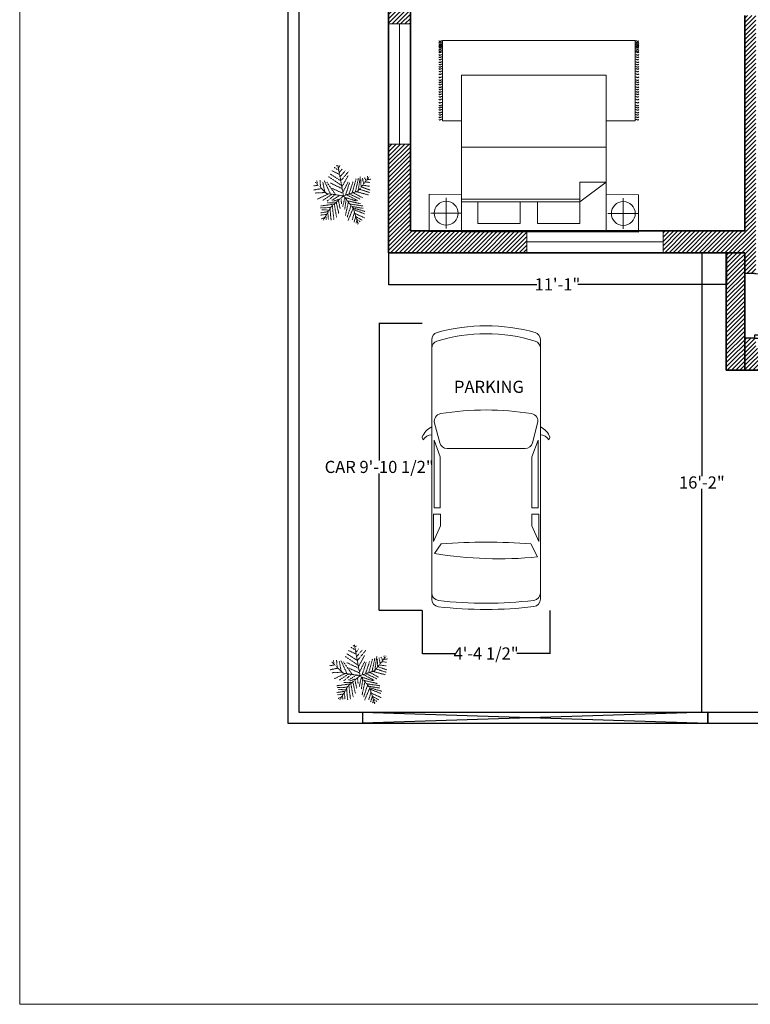
# Model space of a CAD drawing. Units: inches. Extents: x 2202345 to 2203065, y -970921 to -970107.
# Tile 1 of 5: x 2202345 to 2202646, y -970921 to -970515. Entities that reach past the tile are written whole.
import ezdxf

# ---------------------------------------------------------------- set-up
doc = ezdxf.new("R2010")
doc.units = ezdxf.units.IN
doc.header["$MEASUREMENT"] = 0
doc.linetypes.add('HIDDEN', pattern=[0.375, 0.25, -0.125])
doc.layers.get('0').update_dxf_attribs({"color": 13})
for name, color, linetype, lineweight in [('A-ANNO-DIMS', 2, 'Continuous', 18), ('A-ANNO-TTLB', 7, 'HIDDEN', 18), ('A-AREA-IDEN', 7, 'Continuous', 18), ('A-WALL-PATT', 8, 'Continuous', 13), ('C-PROP', 7, 'Continuous', 25), ('doors', 252, 'Continuous', 25), ('furniture', 250, 'Continuous', 18), ('garden', 114, 'HIDDEN', 13), ('gate', 1, 'Continuous', 25), ('parking', 7, 'Continuous', 18), ('PLUMBING FIXTURES', 8, 'Continuous', 18), ('walls', 252, 'Continuous', 35), ('windows', 173, 'Continuous', 18)]:
    doc.layers.add(name, color=color, linetype=linetype, lineweight=lineweight)
doc.styles.get("Standard").update_dxf_attribs({"font": 'arial.ttf'})
doc.dimstyles.get("Standard").update_dxf_attribs({"dimtxt": 5, "dimasz": 0.18, "dimexe": 0.18, "dimexo": 0.0625, "dimgap": 0.09, "dimtad": 0, "dimtih": 1, "dimtoh": 1, "dimzin": 0, "dimdsep": 46, "dimlunit": 3, "dimtxsty": 'Standard', "dimcen": 0.09, "dimadec": 0, "dimazin": 0, "dimtfac": 1, "dimtofl": 0, "dimtmove": 0, "dimatfit": 3, "dimfxl": 1, "dimtolj": 1, "dimtzin": 0, "dimarcsym": 0})
pattern_1 = [(45, (0, 0), (-0.8838834765, 0.8838834765), [])]

# ---------------------------------------------------------------- blocks, each defined once
blk = doc.blocks.new('CARPET')
at = {"layer": 'furniture'}
for p, q in [((-51.53, -98.11), (-51.53, -55.12)), ((-51.53, -55.12), (-41.27, -55.12)), ((36, -55.12), (51.55, -55.12)), ((51.55, -55.12), (51.55, -98.11)), ((51.55, -98.11), (-51.53, -98.11))]:
    blk.add_line(p, q, dxfattribs=at)
for points, knots in [([(-53.37, -55.99), (-53.22, -55.8), (-52.9, -55.41), (-52.34, -55.8), (-51.89, -56.08), (-51.65, -55.91), (-51.53, -55.83)], [0, 0, 0, 0, 0.653278, 1.290138, 1.740457, 2.114451, 2.114451, 2.114451, 2.114451]), ([(-53.37, -57.26), (-53.22, -57.07), (-52.9, -56.67), (-52.34, -57.07), (-51.89, -57.35), (-51.65, -57.17), (-51.53, -57.1)], [0, 0, 0, 0, 0.653278, 1.290138, 1.740457, 2.114451, 2.114451, 2.114451, 2.114451]), ([(53.37, -55.99), (53.22, -55.8), (52.9, -55.41), (52.34, -55.8), (51.89, -56.08), (51.65, -55.91), (51.53, -55.83)], [0, 0, 0, 0, 0.653278, 1.290138, 1.740457, 2.114451, 2.114451, 2.114451, 2.114451]), ([(53.37, -57.26), (53.22, -57.07), (52.9, -56.67), (52.34, -57.07), (51.89, -57.35), (51.65, -57.17), (51.53, -57.1)], [0, 0, 0, 0, 0.653278, 1.290138, 1.740457, 2.114451, 2.114451, 2.114451, 2.114451]), ([(-53.37, -58.59), (-53.22, -58.4), (-52.9, -58.01), (-52.34, -58.4), (-51.89, -58.68), (-51.65, -58.5), (-51.53, -58.43)], [0, 0, 0, 0, 0.653278, 1.290138, 1.740457, 2.114451, 2.114451, 2.114451, 2.114451]), ([(-53.37, -59.78), (-53.22, -59.58), (-52.9, -59.19), (-52.34, -59.58), (-51.89, -59.86), (-51.65, -59.69), (-51.53, -59.61)], [0, 0, 0, 0, 0.653278, 1.290138, 1.740457, 2.114451, 2.114451, 2.114451, 2.114451]), ([(-53.37, -61.22), (-53.22, -61.02), (-52.9, -60.63), (-52.34, -61.02), (-51.89, -61.3), (-51.65, -61.13), (-51.53, -61.05)], [0, 0, 0, 0, 0.653278, 1.290138, 1.740457, 2.114451, 2.114451, 2.114451, 2.114451]), ([(-53.37, -62.44), (-53.22, -62.25), (-52.9, -61.86), (-52.34, -62.25), (-51.89, -62.53), (-51.65, -62.36), (-51.53, -62.28)], [0, 0, 0, 0, 0.653278, 1.290138, 1.740457, 2.114451, 2.114451, 2.114451, 2.114451]), ([(53.37, -58.59), (53.22, -58.4), (52.9, -58.01), (52.34, -58.4), (51.89, -58.68), (51.65, -58.5), (51.53, -58.43)], [0, 0, 0, 0, 0.653278, 1.290138, 1.740457, 2.114451, 2.114451, 2.114451, 2.114451]), ([(53.37, -59.78), (53.22, -59.58), (52.9, -59.19), (52.34, -59.58), (51.89, -59.86), (51.65, -59.69), (51.53, -59.61)], [0, 0, 0, 0, 0.653278, 1.290138, 1.740457, 2.114451, 2.114451, 2.114451, 2.114451]), ([(53.37, -61.22), (53.22, -61.02), (52.9, -60.63), (52.34, -61.02), (51.89, -61.3), (51.65, -61.13), (51.53, -61.05)], [0, 0, 0, 0, 0.653278, 1.290138, 1.740457, 2.114451, 2.114451, 2.114451, 2.114451]), ([(53.37, -62.44), (53.22, -62.25), (52.9, -61.86), (52.34, -62.25), (51.89, -62.53), (51.65, -62.36), (51.53, -62.28)], [0, 0, 0, 0, 0.653278, 1.290138, 1.740457, 2.114451, 2.114451, 2.114451, 2.114451]), ([(-53.37, -63.63), (-53.22, -63.43), (-52.9, -63.04), (-52.34, -63.43), (-51.89, -63.72), (-51.65, -63.54), (-51.53, -63.46)], [0, 0, 0, 0, 0.653278, 1.290138, 1.740457, 2.114451, 2.114451, 2.114451, 2.114451]), ([(-53.37, -65.07), (-53.22, -64.87), (-52.9, -64.48), (-52.34, -64.87), (-51.89, -65.15), (-51.65, -64.98), (-51.53, -64.9)], [0, 0, 0, 0, 0.653278, 1.290138, 1.740457, 2.114451, 2.114451, 2.114451, 2.114451]), ([(-53.37, -66.76), (-53.22, -66.56), (-52.9, -66.17), (-52.34, -66.56), (-51.89, -66.84), (-51.65, -66.67), (-51.53, -66.59)], [0, 0, 0, 0, 0.653278, 1.290138, 1.740457, 2.114451, 2.114451, 2.114451, 2.114451]), ([(-53.37, -68.2), (-53.22, -68), (-52.9, -67.61), (-52.34, -68), (-51.89, -68.28), (-51.65, -68.11), (-51.53, -68.03)], [0, 0, 0, 0, 0.653278, 1.290138, 1.740457, 2.114451, 2.114451, 2.114451, 2.114451]), ([(53.37, -63.63), (53.22, -63.43), (52.9, -63.04), (52.34, -63.43), (51.89, -63.72), (51.65, -63.54), (51.53, -63.46)], [0, 0, 0, 0, 0.653278, 1.290138, 1.740457, 2.114451, 2.114451, 2.114451, 2.114451]), ([(53.37, -65.07), (53.22, -64.87), (52.9, -64.48), (52.34, -64.87), (51.89, -65.15), (51.65, -64.98), (51.53, -64.9)], [0, 0, 0, 0, 0.653278, 1.290138, 1.740457, 2.114451, 2.114451, 2.114451, 2.114451]), ([(53.37, -66.76), (53.22, -66.56), (52.9, -66.17), (52.34, -66.56), (51.89, -66.84), (51.65, -66.67), (51.53, -66.59)], [0, 0, 0, 0, 0.653278, 1.290138, 1.740457, 2.114451, 2.114451, 2.114451, 2.114451]), ([(53.37, -68.2), (53.22, -68), (52.9, -67.61), (52.34, -68), (51.89, -68.28), (51.65, -68.11), (51.53, -68.03)], [0, 0, 0, 0, 0.653278, 1.290138, 1.740457, 2.114451, 2.114451, 2.114451, 2.114451]), ([(-53.37, -69.53), (-53.22, -69.33), (-52.9, -68.94), (-52.34, -69.33), (-51.89, -69.61), (-51.65, -69.44), (-51.53, -69.36)], [0, 0, 0, 0, 0.653278, 1.290138, 1.740457, 2.114451, 2.114451, 2.114451, 2.114451]), ([(-53.37, -70.79), (-53.22, -70.6), (-52.9, -70.21), (-52.34, -70.6), (-51.89, -70.88), (-51.65, -70.7), (-51.53, -70.63)], [0, 0, 0, 0, 0.653278, 1.290138, 1.740457, 2.114451, 2.114451, 2.114451, 2.114451]), ([(-53.37, -72.12), (-53.22, -71.93), (-52.9, -71.54), (-52.34, -71.93), (-51.89, -72.21), (-51.65, -72.04), (-51.53, -71.96)], [0, 0, 0, 0, 0.653278, 1.290138, 1.740457, 2.114451, 2.114451, 2.114451, 2.114451]), ([(-53.37, -73.31), (-53.22, -73.11), (-52.9, -72.72), (-52.34, -73.11), (-51.89, -73.4), (-51.65, -73.22), (-51.53, -73.14)], [0, 0, 0, 0, 0.653278, 1.290138, 1.740457, 2.114451, 2.114451, 2.114451, 2.114451]), ([(53.37, -69.53), (53.22, -69.33), (52.9, -68.94), (52.34, -69.33), (51.89, -69.61), (51.65, -69.44), (51.53, -69.36)], [0, 0, 0, 0, 0.653278, 1.290138, 1.740457, 2.114451, 2.114451, 2.114451, 2.114451]), ([(53.37, -70.79), (53.22, -70.6), (52.9, -70.21), (52.34, -70.6), (51.89, -70.88), (51.65, -70.7), (51.53, -70.63)], [0, 0, 0, 0, 0.653278, 1.290138, 1.740457, 2.114451, 2.114451, 2.114451, 2.114451]), ([(53.37, -72.12), (53.22, -71.93), (52.9, -71.54), (52.34, -71.93), (51.89, -72.21), (51.65, -72.04), (51.53, -71.96)], [0, 0, 0, 0, 0.653278, 1.290138, 1.740457, 2.114451, 2.114451, 2.114451, 2.114451]), ([(53.37, -73.31), (53.22, -73.11), (52.9, -72.72), (52.34, -73.11), (51.89, -73.4), (51.65, -73.22), (51.53, -73.14)], [0, 0, 0, 0, 0.653278, 1.290138, 1.740457, 2.114451, 2.114451, 2.114451, 2.114451]), ([(-53.37, -74.75), (-53.22, -74.55), (-52.9, -74.16), (-52.34, -74.55), (-51.89, -74.83), (-51.65, -74.66), (-51.53, -74.58)], [0, 0, 0, 0, 0.653278, 1.290138, 1.740457, 2.114451, 2.114451, 2.114451, 2.114451]), ([(-53.37, -75.98), (-53.22, -75.78), (-52.9, -75.39), (-52.34, -75.78), (-51.89, -76.06), (-51.65, -75.89), (-51.53, -75.81)], [0, 0, 0, 0, 0.653278, 1.290138, 1.740457, 2.114451, 2.114451, 2.114451, 2.114451]), ([(-53.37, -77.16), (-53.22, -76.96), (-52.9, -76.57), (-52.34, -76.96), (-51.89, -77.25), (-51.65, -77.07), (-51.53, -76.99)], [0, 0, 0, 0, 0.653278, 1.290138, 1.740457, 2.114451, 2.114451, 2.114451, 2.114451]), ([(-53.37, -78.6), (-53.22, -78.4), (-52.9, -78.01), (-52.34, -78.4), (-51.89, -78.68), (-51.65, -78.51), (-51.53, -78.43)], [0, 0, 0, 0, 0.653278, 1.290138, 1.740457, 2.114451, 2.114451, 2.114451, 2.114451]), ([(53.37, -74.75), (53.22, -74.55), (52.9, -74.16), (52.34, -74.55), (51.89, -74.83), (51.65, -74.66), (51.53, -74.58)], [0, 0, 0, 0, 0.653278, 1.290138, 1.740457, 2.114451, 2.114451, 2.114451, 2.114451]), ([(53.37, -75.98), (53.22, -75.78), (52.9, -75.39), (52.34, -75.78), (51.89, -76.06), (51.65, -75.89), (51.53, -75.81)], [0, 0, 0, 0, 0.653278, 1.290138, 1.740457, 2.114451, 2.114451, 2.114451, 2.114451]), ([(53.37, -77.16), (53.22, -76.96), (52.9, -76.57), (52.34, -76.96), (51.89, -77.25), (51.65, -77.07), (51.53, -76.99)], [0, 0, 0, 0, 0.653278, 1.290138, 1.740457, 2.114451, 2.114451, 2.114451, 2.114451]), ([(53.37, -78.6), (53.22, -78.4), (52.9, -78.01), (52.34, -78.4), (51.89, -78.68), (51.65, -78.51), (51.53, -78.43)], [0, 0, 0, 0, 0.653278, 1.290138, 1.740457, 2.114451, 2.114451, 2.114451, 2.114451]), ([(-53.37, -80.29), (-53.22, -80.09), (-52.9, -79.7), (-52.34, -80.09), (-51.89, -80.37), (-51.65, -80.2), (-51.53, -80.12)], [0, 0, 0, 0, 0.653278, 1.290138, 1.740457, 2.114451, 2.114451, 2.114451, 2.114451]), ([(-53.37, -81.73), (-53.22, -81.53), (-52.9, -81.14), (-52.34, -81.53), (-51.89, -81.81), (-51.65, -81.64), (-51.53, -81.56)], [0, 0, 0, 0, 0.653278, 1.290138, 1.740457, 2.114451, 2.114451, 2.114451, 2.114451]), ([(-53.37, -83.06), (-53.22, -82.86), (-52.9, -82.47), (-52.34, -82.86), (-51.89, -83.14), (-51.65, -82.97), (-51.53, -82.89)], [0, 0, 0, 0, 0.653278, 1.290138, 1.740457, 2.114451, 2.114451, 2.114451, 2.114451]), ([(-53.37, -84.18), (-53.22, -83.99), (-52.9, -83.6), (-52.34, -83.99), (-51.89, -84.27), (-51.65, -84.09), (-51.53, -84.02)], [0, 0, 0, 0, 0.653278, 1.290138, 1.740457, 2.114451, 2.114451, 2.114451, 2.114451]), ([(53.37, -80.29), (53.22, -80.09), (52.9, -79.7), (52.34, -80.09), (51.89, -80.37), (51.65, -80.2), (51.53, -80.12)], [0, 0, 0, 0, 0.653278, 1.290138, 1.740457, 2.114451, 2.114451, 2.114451, 2.114451]), ([(53.37, -81.73), (53.22, -81.53), (52.9, -81.14), (52.34, -81.53), (51.89, -81.81), (51.65, -81.64), (51.53, -81.56)], [0, 0, 0, 0, 0.653278, 1.290138, 1.740457, 2.114451, 2.114451, 2.114451, 2.114451]), ([(53.37, -83.06), (53.22, -82.86), (52.9, -82.47), (52.34, -82.86), (51.89, -83.14), (51.65, -82.97), (51.53, -82.89)], [0, 0, 0, 0, 0.653278, 1.290138, 1.740457, 2.114451, 2.114451, 2.114451, 2.114451]), ([(53.37, -84.18), (53.22, -83.99), (52.9, -83.6), (52.34, -83.99), (51.89, -84.27), (51.65, -84.09), (51.53, -84.02)], [0, 0, 0, 0, 0.653278, 1.290138, 1.740457, 2.114451, 2.114451, 2.114451, 2.114451]), ([(-53.37, -85.51), (-53.22, -85.32), (-52.9, -84.93), (-52.34, -85.32), (-51.89, -85.6), (-51.65, -85.42), (-51.53, -85.35)], [0, 0, 0, 0, 0.653278, 1.290138, 1.740457, 2.114451, 2.114451, 2.114451, 2.114451]), ([(-53.37, -86.7), (-53.22, -86.5), (-52.9, -86.11), (-52.34, -86.5), (-51.89, -86.78), (-51.65, -86.61), (-51.53, -86.53)], [0, 0, 0, 0, 0.653278, 1.290138, 1.740457, 2.114451, 2.114451, 2.114451, 2.114451]), ([(-53.37, -88.14), (-53.22, -87.94), (-52.9, -87.55), (-52.34, -87.94), (-51.89, -88.22), (-51.65, -88.05), (-51.53, -87.97)], [0, 0, 0, 0, 0.653278, 1.290138, 1.740457, 2.114451, 2.114451, 2.114451, 2.114451]), ([(-53.37, -89.36), (-53.22, -89.17), (-52.9, -88.78), (-52.34, -89.17), (-51.89, -89.45), (-51.65, -89.28), (-51.53, -89.2)], [0, 0, 0, 0, 0.653278, 1.290138, 1.740457, 2.114451, 2.114451, 2.114451, 2.114451]), ([(53.37, -85.51), (53.22, -85.32), (52.9, -84.93), (52.34, -85.32), (51.89, -85.6), (51.65, -85.42), (51.53, -85.35)], [0, 0, 0, 0, 0.653278, 1.290138, 1.740457, 2.114451, 2.114451, 2.114451, 2.114451]), ([(53.37, -86.7), (53.22, -86.5), (52.9, -86.11), (52.34, -86.5), (51.89, -86.78), (51.65, -86.61), (51.53, -86.53)], [0, 0, 0, 0, 0.653278, 1.290138, 1.740457, 2.114451, 2.114451, 2.114451, 2.114451]), ([(53.37, -88.14), (53.22, -87.94), (52.9, -87.55), (52.34, -87.94), (51.89, -88.22), (51.65, -88.05), (51.53, -87.97)], [0, 0, 0, 0, 0.653278, 1.290138, 1.740457, 2.114451, 2.114451, 2.114451, 2.114451]), ([(53.37, -89.36), (53.22, -89.17), (52.9, -88.78), (52.34, -89.17), (51.89, -89.45), (51.65, -89.28), (51.53, -89.2)], [0, 0, 0, 0, 0.653278, 1.290138, 1.740457, 2.114451, 2.114451, 2.114451, 2.114451]), ([(-53.37, -90.55), (-53.22, -90.35), (-52.9, -89.96), (-52.34, -90.35), (-51.89, -90.64), (-51.65, -90.46), (-51.53, -90.38)], [0, 0, 0, 0, 0.653278, 1.290138, 1.740457, 2.114451, 2.114451, 2.114451, 2.114451]), ([(-53.37, -91.99), (-53.22, -91.79), (-52.9, -91.4), (-52.34, -91.79), (-51.89, -92.07), (-51.65, -91.9), (-51.53, -91.82)], [0, 0, 0, 0, 0.653278, 1.290138, 1.740457, 2.114451, 2.114451, 2.114451, 2.114451]), ([(-53.37, -92.69), (-53.22, -92.48), (-52.9, -92.08), (-52.35, -92.49), (-51.89, -92.77), (-51.65, -92.6), (-51.53, -92.52)], [0, 0, 0, 0, 0.663904, 1.307406, 1.757725, 2.131719, 2.131719, 2.131719, 2.131719]), ([(-53.37, -93.61), (-53.22, -93.42), (-52.9, -93.03), (-52.34, -93.42), (-51.89, -93.7), (-51.65, -93.52), (-51.53, -93.45)], [0, 0, 0, 0, 0.653278, 1.290138, 1.740457, 2.114451, 2.114451, 2.114451, 2.114451]), ([(-53.37, -94.55), (-53.22, -94.35), (-52.9, -93.96), (-52.34, -94.35), (-51.89, -94.63), (-51.65, -94.46), (-51.53, -94.38)], [0, 0, 0, 0, 0.653278, 1.290138, 1.740457, 2.114451, 2.114451, 2.114451, 2.114451]), ([(-53.37, -95.05), (-53.22, -94.85), (-52.9, -94.46), (-52.34, -94.85), (-51.89, -95.14), (-51.65, -94.96), (-51.53, -94.88)], [0, 0, 0, 0, 0.653278, 1.290138, 1.740457, 2.114451, 2.114451, 2.114451, 2.114451]), ([(53.37, -90.55), (53.22, -90.35), (52.9, -89.96), (52.34, -90.35), (51.9, -90.63), (51.66, -90.47), (51.55, -90.4)], [0, 0, 0, 0, 0.653278, 1.290138, 1.740457, 2.0926, 2.0926, 2.0926, 2.0926]), ([(53.37, -91.99), (53.22, -91.79), (52.9, -91.4), (52.34, -91.79), (51.9, -92.07), (51.66, -91.91), (51.55, -91.83)], [0, 0, 0, 0, 0.653278, 1.290138, 1.740457, 2.0926, 2.0926, 2.0926, 2.0926]), ([(53.37, -92.69), (53.22, -92.49), (52.9, -92.09), (52.34, -92.49), (51.9, -92.77), (51.66, -92.61), (51.55, -92.53)], [0, 0, 0, 0, 0.656792, 1.295826, 1.746145, 2.098292, 2.098292, 2.098292, 2.098292]), ([(53.37, -93.66), (53.22, -93.46), (52.9, -93.07), (52.34, -93.46), (51.9, -93.74), (51.66, -93.58), (51.55, -93.5)], [0, 0, 0, 0, 0.653278, 1.290138, 1.740457, 2.0926, 2.0926, 2.0926, 2.0926]), ([(53.37, -94.59), (53.22, -94.4), (52.9, -94.01), (52.34, -94.4), (51.9, -94.68), (51.66, -94.51), (51.55, -94.44)], [0, 0, 0, 0, 0.653278, 1.290138, 1.740457, 2.0926, 2.0926, 2.0926, 2.0926]), ([(-53.37, -95.73), (-53.22, -95.54), (-52.9, -95.15), (-52.34, -95.54), (-51.89, -95.82), (-51.65, -95.65), (-51.53, -95.57)], [0, 0, 0, 0, 0.653278, 1.290138, 1.740457, 2.114451, 2.114451, 2.114451, 2.114451]), ([(-53.37, -96.38), (-53.22, -96.18), (-52.9, -95.79), (-52.34, -96.18), (-51.89, -96.47), (-51.65, -96.29), (-51.53, -96.21)], [0, 0, 0, 0, 0.653278, 1.290138, 1.740457, 2.114451, 2.114451, 2.114451, 2.114451]), ([(-53.37, -97.17), (-53.22, -96.98), (-52.9, -96.59), (-52.34, -96.98), (-51.89, -97.26), (-51.65, -97.08), (-51.53, -97.01)], [0, 0, 0, 0, 0.653278, 1.290138, 1.740457, 2.114451, 2.114451, 2.114451, 2.114451]), ([(-53.37, -97.99), (-53.22, -97.79), (-52.9, -97.4), (-52.34, -97.79), (-51.89, -98.08), (-51.65, -97.9), (-51.53, -97.82)], [0, 0, 0, 0, 0.653278, 1.290138, 1.740457, 2.114451, 2.114451, 2.114451, 2.114451]), ([(53.37, -95.78), (53.22, -95.58), (52.9, -95.19), (52.34, -95.58), (51.89, -95.86), (51.65, -95.69), (51.53, -95.61)], [0, 0, 0, 0, 0.653278, 1.290138, 1.740457, 2.114451, 2.114451, 2.114451, 2.114451]), ([(53.37, -96.43), (53.22, -96.23), (52.9, -95.84), (52.34, -96.23), (51.89, -96.51), (51.65, -96.34), (51.53, -96.26)], [0, 0, 0, 0, 0.653278, 1.290138, 1.740457, 2.114451, 2.114451, 2.114451, 2.114451]), ([(53.37, -97.22), (53.22, -97.02), (52.9, -96.63), (52.34, -97.02), (51.89, -97.3), (51.65, -97.13), (51.53, -97.05)], [0, 0, 0, 0, 0.653278, 1.290138, 1.740457, 2.114451, 2.114451, 2.114451, 2.114451]), ([(53.37, -97.99), (53.22, -97.79), (52.9, -97.4), (52.34, -97.79), (51.89, -98.08), (51.65, -97.9), (51.53, -97.82)], [0, 0, 0, 0, 0.653278, 1.290138, 1.740457, 2.114451, 2.114451, 2.114451, 2.114451]), ([(53.37, -95.1), (53.22, -94.9), (52.9, -94.51), (52.34, -94.9), (51.9, -95.18), (51.66, -95.02), (51.55, -94.94)], [0, 0, 0, 0, 0.653278, 1.290138, 1.740457, 2.0926, 2.0926, 2.0926, 2.0926])]:
    blk.add_open_spline(points, degree=3, knots=knots, dxfattribs=at)
blk = doc.blocks.new('A$C58D270C6')
at = {"layer": 'furniture'}
for p, q in [((9.09, 124.13), (9.09, 108.87)), ((1.46, 116.5), (16.73, 116.5)), ((14.97, 94.84), (24.62, 107.92)), ((24.62, 94.93), (24.62, 107.92)), ((42.08, 108), (42.08, 36)), ((14.97, 94.93), (24.62, 94.93)), ((14.97, 94.84), (14.97, 36)), ((16.22, 94.93), (16.22, 36)), ((9.25, 36), (9.25, 20.74)), ((1.62, 28.37), (16.88, 28.37))]:
    blk.add_line(p, q, dxfattribs=at)
for points in [[(18.5, 108), (18.34, 124.13), (-0.16, 124.13), (0, 108)], [(0, 108), (77.91, 108), (77.91, 36), (0, 36)], [(4.09, 94.93), (14.97, 94.93), (14.97, 73.83), (4.09, 73.83)], [(4.09, 65.23), (14.97, 65.23), (14.97, 44.13), (4.09, 44.13)], [(18.65, 19.87), (18.5, 36), (0, 36), (0.16, 19.87)]]:
    blk.add_lwpolyline(points, close=True, dxfattribs=at)
for centre in [(9.09, 116.5), (9.25, 28.37)]:
    blk.add_circle(centre, 5.95, dxfattribs=at)
at = {"layer": 'furniture', "xscale": 0.9312884925094044, "yscale": 0.9312884925094044, "zscale": 0.9312884925094044, "rotation": 90}
blk.add_blockref('CARPET', (3.79, 74.47), dxfattribs=at)
blk = doc.blocks.new('*U12')
for p, q in [((0, 0), (0, -6)), ((40, 0), (40, -6))]:
    blk.add_line(p, q)
blk.add_lwpolyline([(0, 0), (0, 40), (1.75, 40), (1.75, 0)], close=True)
blk.add_arc((0, 0), 40, 0, 90)
blk = doc.blocks.new('CAR')
at = {"layer": 'PLUMBING FIXTURES', "ltscale": 3}
for p, q in [((220804.47, -93720.06), (220804.47, -93547.3)), ((220876.86, -93720.06), (220876.86, -93547.35)), ((220870.5, -93584.17), (220875, -93575.44)), ((220810.83, -93584.17), (220806.31, -93577.76)), ((220810.23, -93596.08), (220805.58, -93585.68)), ((220805.58, -93585.68), (220805.58, -93603.85)), ((220871.11, -93596.08), (220875.75, -93585.68)), ((220875.75, -93585.68), (220875.75, -93603.85)), ((220810.23, -93603.85), (220810.23, -93596.08)), ((220871.11, -93603.85), (220871.11, -93596.08)), ((220805.58, -93603.85), (220810.23, -93603.85)), ((220805.99, -93608.09), (220810.13, -93608.09)), ((220805.99, -93653.29), (220805.99, -93608.09)), ((220810.13, -93608.09), (220810.13, -93642.08)), ((220875.75, -93603.85), (220871.11, -93603.85)), ((220875.35, -93608.09), (220871.21, -93608.09)), ((220871.21, -93608.09), (220871.21, -93642.08)), ((220875.35, -93653.29), (220875.35, -93608.09)), ((220810.13, -93642.08), (220805.99, -93653.29)), ((220871.21, -93642.08), (220875.35, -93653.29)), ((220814.66, -93647.63), (220866.67, -93647.63)), ((220798.82, -93653.49), (220798.11, -93655.1)), ((220806.3, -93664.61), (220809.78, -93651.39)), ((220875.03, -93664.61), (220871.56, -93651.39)), ((220882.52, -93653.49), (220883.22, -93655.1))]:
    blk.add_line(p, q, dxfattribs=at)
for centre, radius, start, end in [((220809.52, -93547.3), 5.05, 97.35661, 179.99999), ((220840.49, -93811.75), 271.3, 83.23106, 96.6925), ((220840.49, -93815.88), 271.3, 83.23106, 96.6925), ((220871.81, -93547.35), 5.05, 359.99999, 82.55935), ((220809.52, -93551.44), 5.05, 97.35661, 179.99999), ((220871.81, -93551.49), 5.05, 359.99999, 82.55935), ((220849.45, -93836.99), 262.8, 84.42019, 99.44802), ((220840.67, -93184.08), 401.19, 265.73533, 274.26465), ((220814.66, -93652.68), 5.05, 89.99999, 165.25643), ((220866.67, -93652.68), 5.05, 14.74356, 89.99999), ((220809.44, -93651.03), 12.03, 199.79435, 245.64582), ((220804.88, -93649.65), 7.17, 212.34744, 266.77131), ((220876.46, -93649.65), 7.17, 273.22867, 327.65255), ((220871.9, -93651.03), 12.03, 294.35417, 340.20564), ((220811.18, -93665.89), 5.05, 165.25643, 260.06484), ((220870.15, -93665.89), 5.05, 279.93514, 14.74356), ((220840.67, -93484.81), 188.52, 260.73418, 279.2658), ((220809.52, -93714.44), 5.05, 179.99999, 251.46365), ((220871.81, -93714.44), 5.05, 288.53634, 359.99999), ((220809.52, -93720.06), 5.05, 179.99999, 252.55068), ((220840.67, -93611.64), 112.45, 253.06746, 286.93252), ((220871.81, -93720.06), 5.05, 287.4493, 359.99999), ((220840.67, -93610.47), 118.98, 254.06731, 285.93267)]:
    blk.add_arc(centre, radius, start, end, dxfattribs=at)
blk = doc.blocks.new('*D15')
at = {"layer": 'A-ANNO-DIMS', "color": 0, "lineweight": -2, "transparency": 16777216}
for p, q in [((2202496.68, -970610.67), (2202496.68, -970623.86)), ((2202636.04, -970610.67), (2202636.04, -970623.86)), ((2202496.86, -970623.68), (2202557.92, -970623.68)), ((2202635.86, -970623.68), (2202574.8, -970623.68))]:
    blk.add_line(p, q, dxfattribs=at)
at = {"layer": 'A-ANNO-DIMS', "color": 0, "transparency": 16777216}
for points in [[(2202496.86, -970623.65), (2202496.86, -970623.71), (2202496.68, -970623.68)], [(2202635.86, -970623.65), (2202635.86, -970623.71), (2202636.04, -970623.68)]]:
    blk.add_solid(points, dxfattribs=at)
at = {"layer": 'Defpoints', "color": 0, "transparency": 16777216}
for p in [(2202496.68, -970610.61), (2202636.04, -970610.61), (2202636.04, -970623.68)]:
    blk.add_point(p, dxfattribs=at)
at = {"layer": 'A-ANNO-DIMS', "color": 0, "transparency": 16777216, "insert": (2202566.36, -970623.68), "char_height": 5, "attachment_point": 5}
blk.add_mtext('\\A1;11\'-1"', dxfattribs=at)
blk = doc.blocks.new('*D16')
at = {"layer": 'A-ANNO-DIMS', "color": 0, "lineweight": -2, "transparency": 16777216}
for p, q in [((2202621.98, -970610.61), (2202626.13, -970610.61)), ((2202625.95, -970610.79), (2202625.95, -970702.71)), ((2202625.95, -970799.93), (2202625.95, -970708)), ((2202621.98, -970800.11), (2202626.13, -970800.11))]:
    blk.add_line(p, q, dxfattribs=at)
at = {"layer": 'A-ANNO-DIMS', "color": 0, "transparency": 16777216}
for points in [[(2202625.92, -970610.79), (2202625.98, -970610.79), (2202625.95, -970610.61)], [(2202625.92, -970799.93), (2202625.98, -970799.93), (2202625.95, -970800.11)]]:
    blk.add_solid(points, dxfattribs=at)
at = {"layer": 'Defpoints', "color": 0, "transparency": 16777216}
for p in [(2202621.91, -970610.61), (2202621.91, -970800.11), (2202625.95, -970800.11)]:
    blk.add_point(p, dxfattribs=at)
at = {"layer": 'A-ANNO-DIMS', "color": 0, "transparency": 16777216, "insert": (2202625.95, -970705.36), "char_height": 5, "attachment_point": 5}
blk.add_mtext('\\A1;16\'-2"', dxfattribs=at)
blk = doc.blocks.new('*U23')
for p, q in [((-10.186, 53.64), (-13.084, 55.962)), ((0, 0), (-10.5, 57)), ((-9.099, 51.782), (-6.563, 55.962)), ((-5.114, 28.097), (-24.676, 40.636)), ((-7.288, 39.707), (-21.778, 46.673)), ((-8.737, 47.138), (-17.069, 52.711)), ((-7.65, 43.423), (-2.578, 49.46)), ((-5.839, 35.992), (4.667, 48.067)), ((-5.114, 27.632), (10.463, 46.673)), ((-2.941, 16.486), (8.652, 37.85)), ((44.153, 36.456), (45.239, 32.741)), ((-47.498, 19.737), (-55.83, 18.344)), ((-31.5, 4.5), (-52.5, 25.5)), ((-48.585, 21.131), (-49.309, 29.026)), ((-43.513, 28.561), (-42.427, 15.558)), ((-38.442, 26.239), (-34.819, 7.663)), ((-35.544, 28.097), (-24.314, 3.947)), ((-14.533, 2.09), (-30.834, 25.31)), ((-3.665, 19.273), (-27.574, 35.527)), ((-24.314, 23.917), (-2.941, 13.7)), ((-1.129, 6.734), (9.014, 26.704)), ((3.942, 1.625), (11.187, 24.381)), ((10.101, 3.483), (17.708, 26.239)), ((16.259, 5.805), (23.142, 31.348)), ((22.055, 7.198), (27.489, 32.277)), ((27, 9), (48, 36)), ((27.127, 9.056), (31.112, 35.992)), ((31.836, 30.883), (32.561, 16.486)), ((35.096, 32.741), (37.27, 22.524)), ((36.183, 19.737), (48.137, 17.88)), ((38.719, 34.134), (41.979, 28.561)), ((40.53, 25.775), (48.862, 24.846)), ((43.791, 29.954), (51.036, 30.883)), ((-40.615, 13.7), (-55.105, 10.913)), ((-33.37, 6.269), (-52.207, 5.34)), ((-28.299, 3.483), (-47.86, -5.805)), ((-21.416, 3.018), (-38.079, -8.128)), ((0, 0), (-31.5, 4.5)), ((-15.982, 2.09), (-30.11, -9.521)), ((0, 0), (-22.5, -19.5)), ((-6.563, 1.161), (-21.416, -8.128)), ((-20.691, 13.7), (-1.129, 4.876)), ((0, 0), (27, 9)), ((0, 0), (18, -22.5)), ((6.478, 1.625), (26.04, -8.592)), ((11.187, 3.483), (30.749, -5.805)), ((18.07, 5.805), (35.096, -3.483)), ((24.229, 7.663), (46.688, 1.625)), ((29.662, 12.307), (48.137, 6.269)), ((33.285, 16.486), (48.862, 10.913)), ((-17.431, -15.094), (-42.789, -18.809)), ((-15.257, -12.772), (-30.11, -12.772)), ((-6.563, -5.805), (-19.967, -9.985)), ((-17.069, -15.094), (-12.721, -40.172)), ((-13.446, -11.378), (-8.737, -32.741)), ((-9.461, -8.592), (-6.201, -23.453)), ((-4.752, -3.483), (-3.665, -14.629)), ((2.493, -3.019), (-1.491, -20.202)), ((1.769, -2.555), (24.229, -9.521)), ((5.029, -6.27), (2.131, -25.775)), ((9.014, -11.378), (3.58, -35.992)), ((14.085, -16.951), (6.478, -40.172)), ((7.565, -9.056), (32.198, -14.629)), ((12.274, -15.094), (36.907, -18.809)), ((-28.299, -29.026), (-42.789, -31.348)), ((-24.314, -21.596), (-42.427, -22.06)), ((-30.834, -34.135), (-42.427, -35.528)), ((-26.849, -26.24), (-40.253, -25.775)), ((-22.5, -19.5), (-37.5, -45)), ((-29.023, -30.884), (-27.936, -43.887)), ((-25.038, -23.918), (-22.865, -45.281)), ((-20.691, -18.345), (-17.793, -44.352)), ((18.07, -22.524), (8.289, -45.745)), ((20.244, -30.419), (15.897, -44.816)), ((16.259, -19.738), (36.183, -22.989)), ((18, -22.5), (27, -52.5)), ((18.433, -22.524), (40.53, -29.026)), ((19.157, -25.311), (38.719, -33.206)), ((21.331, -32.741), (39.081, -40.636)), ((-34.457, -39.708), (-40.978, -42.494)), ((-32.646, -36.921), (-31.921, -44.352)), ((22.78, -37.85), (19.519, -48.532)), ((22.78, -38.314), (34.372, -44.816)), ((24.591, -45.745), (23.142, -50.854)), ((24.591, -43.423), (30.749, -47.603)), ((26.764, -49.925), (28.213, -50.854))]:
    blk.add_line(p, q)
blk = doc.blocks.new('*D39')
at = {"layer": 'A-ANNO-DIMS', "color": 0, "lineweight": -2, "transparency": 16777216}
for p, q in [((2202510.52, -970639.77), (2202492.65, -970639.77)), ((2202492.83, -970639.95), (2202492.83, -970696.27)), ((2202492.83, -970757.94), (2202492.83, -970701.62)), ((2202510.52, -970758.12), (2202492.65, -970758.12))]:
    blk.add_line(p, q, dxfattribs=at)
at = {"layer": 'A-ANNO-DIMS', "color": 0, "transparency": 16777216}
for points in [[(2202492.8, -970639.95), (2202492.86, -970639.95), (2202492.83, -970639.77)], [(2202492.8, -970757.94), (2202492.86, -970757.94), (2202492.83, -970758.12)]]:
    blk.add_solid(points, dxfattribs=at)
at = {"layer": 'Defpoints', "color": 0, "transparency": 16777216}
for p in [(2202510.58, -970639.77), (2202492.83, -970758.12), (2202510.58, -970758.12)]:
    blk.add_point(p, dxfattribs=at)
at = {"layer": 'A-ANNO-DIMS', "color": 0, "transparency": 16777216, "insert": (2202492.83, -970698.95), "char_height": 5, "attachment_point": 5}
blk.add_mtext('\\A1;CAR 9\'-10 1/2"', dxfattribs=at)
blk = doc.blocks.new('*D40')
at = {"layer": 'A-ANNO-DIMS', "color": 0, "lineweight": -2, "transparency": 16777216}
for p, q in [((2202510.58, -970758.18), (2202510.58, -970776.05)), ((2202563.27, -970758.18), (2202563.27, -970776.05)), ((2202510.76, -970775.87), (2202524.26, -970775.87)), ((2202563.09, -970775.87), (2202549.59, -970775.87))]:
    blk.add_line(p, q, dxfattribs=at)
at = {"layer": 'A-ANNO-DIMS', "color": 0, "transparency": 16777216}
for points in [[(2202510.76, -970775.84), (2202510.76, -970775.9), (2202510.58, -970775.87)], [(2202563.09, -970775.84), (2202563.09, -970775.9), (2202563.27, -970775.87)]]:
    blk.add_solid(points, dxfattribs=at)
at = {"layer": 'Defpoints', "color": 0, "transparency": 16777216}
for p in [(2202510.58, -970758.12), (2202563.27, -970758.12), (2202563.27, -970775.87)]:
    blk.add_point(p, dxfattribs=at)
at = {"layer": 'A-ANNO-DIMS', "color": 0, "transparency": 16777216, "insert": (2202536.93, -970775.87), "char_height": 5, "attachment_point": 5}
blk.add_mtext('\\A1;4\'-4 1/2"', dxfattribs=at)

msp = doc.modelspace()

# ---------------------------------------------------------------- hatches: boundary and pattern name
at = {"layer": 'A-WALL-PATT'}
h = msp.add_hatch(dxfattribs=at)
h.set_pattern_fill('ANSI31', color=256, scale=10)
h.set_pattern_definition(pattern_1)
h.paths.add_polyline_path([(2202648.182, -970512.768), (2202644.707, -970512.768, -0.0110733), (2202643.682, -970512.746), (2202643.682, -970601.606), (2202609.913, -970601.606), (2202609.913, -970610.606), (2202643.682, -970610.606), (2202643.682, -970619.168), (2202647.677, -970619.168, -0.0047326), (2202648.182, -970619.173)])
h.paths.add_polyline_path([(2202643.682, -970610.606), (2202636.037, -970610.606), (2202636.037, -970659.106), (2202643.682, -970659.106)])
h.paths.add_polyline_path([(2202722.39, -970654.606), (2202722.39, -970650.106), (2202648.182, -970650.106), (2202648.182, -970645.806), (2202647.677, -970645.806), (2202643.682, -970645.806), (2202643.682, -970659.106), (2202722.39, -970659.106)])
h.paths.add_polyline_path([(2202846.182, -970650.106), (2202798.148, -970650.106), (2202798.148, -970659.106), (2202846.182, -970659.106)])
h.paths.add_polyline_path([(2202855.182, -970619.995), (2202846.182, -970619.995), (2202846.182, -970682.124), (2202855.182, -970682.124)])
h.paths.add_polyline_path([(2202855.182, -970434.646), (2202846.182, -970434.646), (2202846.182, -970545.038), (2202855.182, -970545.038)])
h.paths.add_polyline_path([(2202903.182, -970745.106), (2202855.182, -970745.106), (2202855.182, -970729.208), (2202846.182, -970729.208), (2202846.182, -970745.106), (2202725.91, -970745.106), (2202725.91, -970754.106), (2202903.182, -970754.106)])
h.paths.add_polyline_path([(2202846.182, -970489.606), (2202767.486, -970489.606, -0.1570508), (2202766.685, -970489.864), (2202739.229, -970489.864, -0.1570508), (2202738.428, -970489.606), (2202685.343, -970489.606), (2202685.343, -970494.106), (2202846.182, -970494.106)])
h.paths.add_polyline_path([(2202648.182, -970477.106), (2202594.182, -970477.106), (2202594.182, -970352.606), (2202624.243, -970352.606), (2202624.243, -970348.106), (2202575.482, -970348.106), (2202575.482, -970352.606), (2202589.682, -970352.606), (2202589.682, -970412.606), (2202505.682, -970412.606), (2202505.682, -970417.106), (2202589.682, -970417.106), (2202589.682, -970477.106), (2202580.925, -970477.106), (2202580.925, -970481.606), (2202643.682, -970481.606), (2202643.682, -970489.606), (2202644.707, -970489.606), (2202648.182, -970489.606)])
h.paths.add_polyline_path([(2202505.682, -970305.515), (2202496.682, -970305.515), (2202496.682, -970378.877), (2202501.298, -970378.877), (2202505.682, -970378.877)])
h.paths.add_polyline_path([(2202540.998, -970348.106), (2202505.682, -970348.106), (2202505.682, -970352.606), (2202540.998, -970352.606)], flags=17)
h.paths.add_polyline_path([(2202505.682, -970452.918), (2202496.682, -970452.918), (2202496.682, -970516.267), (2202505.682, -970516.267)])
h.paths.add_polyline_path([(2202505.682, -970210.106), (2202898.682, -970210.106), (2202898.682, -970294.106), (2202889.459, -970294.106), (2202889.459, -970303.106), (2202907.682, -970303.106), (2202907.682, -970201.106), (2202496.682, -970201.106), (2202496.682, -970242.728), (2202505.682, -970242.728)])
h.paths.add_polyline_path([(2202678.182, -970210.106), (2202673.682, -970210.106), (2202673.682, -970348.106), (2202664.243, -970348.106), (2202664.243, -970352.606), (2202686.569, -970352.606), (2202686.569, -970348.106), (2202678.182, -970348.106)])
h.paths.add_polyline_path([(2202752.572, -970321.843), (2202794.204, -970321.843), (2202794.204, -970314.185), (2202752.572, -970314.185)], flags=9)
h.paths.add_polyline_path([(2202750.562, -970312.127), (2202793.125, -970312.127), (2202793.125, -970304.366), (2202750.562, -970304.366)], flags=9)
h = msp.add_hatch(dxfattribs=at)
h.set_pattern_fill('ANSI31', color=256, scale=10)
h.set_pattern_definition(pattern_1)
h.paths.add_polyline_path([(2202540.925, -970477.106), (2202505.682, -970477.106), (2202505.682, -970481.606), (2202540.925, -970481.606)])
h.paths.add_polyline_path([(2202553.677, -970601.606), (2202505.682, -970601.606), (2202505.682, -970565.796), (2202496.682, -970565.796), (2202496.682, -970610.606), (2202553.677, -970610.606), (2202553.677, -970606.106)])

# ---------------------------------------------------------------- linework, layer by layer
at = {"layer": 'A-ANNO-TTLB'}
for p, q in [((2202344.52, -970106.63), (2202344.52, -970920.555)), ((2202344.52, -970920.555), (2203064.943, -970920.555))]:
    msp.add_line(p, q, dxfattribs=at)
at = {"layer": 'C-PROP'}
for p, q in [((2202455.182, -970201.106), (2202455.182, -970804.606)), ((2202459.682, -970205.606), (2202459.682, -970800.106)), ((2202459.682, -970800.106), (2202903.182, -970800.106)), ((2202455.182, -970804.606), (2202459.682, -970804.606)), ((2202459.682, -970804.606), (2202907.682, -970804.606))]:
    msp.add_line(p, q, dxfattribs=at)
at = {"layer": 'gate'}
for p, q in [((2202485.905, -970800.106), (2202485.905, -970804.606)), ((2202485.905, -970800.106), (2202485.905, -970804.606)), ((2202485.905, -970800.106), (2202628.444, -970804.606)), ((2202628.444, -970800.106), (2202485.905, -970804.606)), ((2202628.444, -970800.106), (2202628.444, -970804.606)), ((2202628.444, -970804.606), (2202628.444, -970800.106))]:
    msp.add_line(p, q, dxfattribs=at)
at = {"layer": 'walls'}
for p, q in [((2202496.682, -970201.106), (2202496.682, -970610.606)), ((2202505.682, -970210.106), (2202505.682, -970601.606)), ((2202643.682, -970512.746), (2202643.682, -970601.606)), ((2202505.682, -970601.606), (2202643.682, -970601.606)), ((2202496.682, -970610.606), (2202643.682, -970610.606)), ((2202636.037, -970610.606), (2202636.037, -970659.106)), ((2202643.682, -970610.606), (2202643.682, -970659.106)), ((2202636.037, -970659.106), (2202643.682, -970659.106)), ((2202643.682, -970659.106), (2202846.182, -970659.106))]:
    msp.add_line(p, q, dxfattribs=at)
at = {"layer": 'windows'}
for p, q in [((2202496.682, -970516.267), (2202505.682, -970516.267)), ((2202505.682, -970516.267), (2202501.182, -970516.267)), ((2202501.182, -970516.267), (2202501.182, -970565.796)), ((2202501.182, -970565.796), (2202496.682, -970565.796)), ((2202496.682, -970565.796), (2202505.682, -970565.796)), ((2202553.677, -970601.606), (2202553.677, -970610.606)), ((2202609.913, -970606.106), (2202609.913, -970601.606)), ((2202609.913, -970601.606), (2202609.913, -970610.606)), ((2202553.677, -970610.606), (2202553.677, -970606.106)), ((2202553.677, -970606.106), (2202609.913, -970606.106))]:
    msp.add_line(p, q, dxfattribs=at)

# ---------------------------------------------------------------- block references
at = {"layer": 'doors', "xscale": -0.6659591083613691, "yscale": 0.6659591083613691, "zscale": 0.6659591083613691, "rotation": 270}
msp.add_blockref('*U12', (2202647.677, -970645.806), dxfattribs=at)
at = {"layer": 'furniture', "xscale": -0.8292897843380787, "yscale": 0.8292897843380787, "zscale": 0.8292897843380787, "rotation": 270}
msp.add_blockref('A$C58D270C6', (2202496.92, -970601.993), dxfattribs=at)
at = {"layer": 'garden', "xscale": 0.2228486455557245, "yscale": 0.2228486455557245, "zscale": 0.2228486455557245}
for p in [(2202478.107, -970587.183), (2202484.946, -970785.007)]:
    msp.add_blockref('*U23', p, dxfattribs=at)
at = {"layer": 'parking', "xscale": -0.6191396643141144, "yscale": 0.6191396643141144, "zscale": 0.6191396643141144, "rotation": 180}
msp.add_blockref('CAR', (2065805.709, -1028672.333), dxfattribs=at)

# ---------------------------------------------------------------- texts
at = {"layer": 'A-AREA-IDEN'}
msp.add_text('PARKING', height=5, dxfattribs=at).set_placement((2202523.678, -970668.404))

# ---------------------------------------------------------------- dimensions: what is measured, and where the dimension line sits
at = {"layer": 'A-ANNO-DIMS'}
dim = msp.add_linear_dim(base=(2202636.037, -970623.678), p1=(2202496.682, -970610.606), p2=(2202636.037, -970610.606), text='11\'-1"', dimstyle='Standard', override={"dimclrd": 0, "dimclre": 0, "dimclrt": 0}, dxfattribs=at)
dim.commit()
dim.dimension.update_dxf_attribs({"geometry": '*D15', "text_midpoint": (2202566.359, -970623.678)})
for base, p1, p2, angle, text, override, picture, middle in [((2202625.945, -970800.106), (2202621.913, -970610.606), (2202621.913, -970800.106), 90, '16\'-2"', {"dimclrd": 0, "dimclre": 0, "dimclrt": 0}, '*D16', (2202625.945, -970705.356)), ((2202492.826, -970758.121), (2202510.578, -970639.77), (2202510.578, -970758.121), 270, 'CAR <>', {"dimdec": 1, "dimlfac": 1, "dimrnd": 0, "dimzin": 1, "dimdsep": 46, "dimlunit": 4, "dimfrac": 2}, '*D39', (2202492.826, -970698.945))]:
    dim = msp.add_linear_dim(base=base, p1=p1, p2=p2, angle=angle, text=text, dimstyle='Standard', override=override, dxfattribs=at)
    dim.commit()
    dim.dimension.update_dxf_attribs({"geometry": picture, "text_midpoint": middle})
dim = msp.add_linear_dim(base=(2202563.274, -970775.874), p1=(2202510.578, -970758.121), p2=(2202563.274, -970758.121), dimstyle='Standard', override={"dimdec": 1, "dimlfac": 1, "dimrnd": 0, "dimzin": 1, "dimdsep": 46, "dimlunit": 4, "dimfrac": 2}, dxfattribs=at)
dim.commit()
dim.dimension.update_dxf_attribs({"geometry": '*D40', "text_midpoint": (2202536.926, -970775.874)})

doc.saveas('drawing.dxf')
